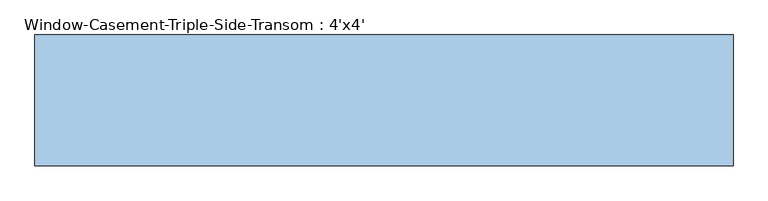
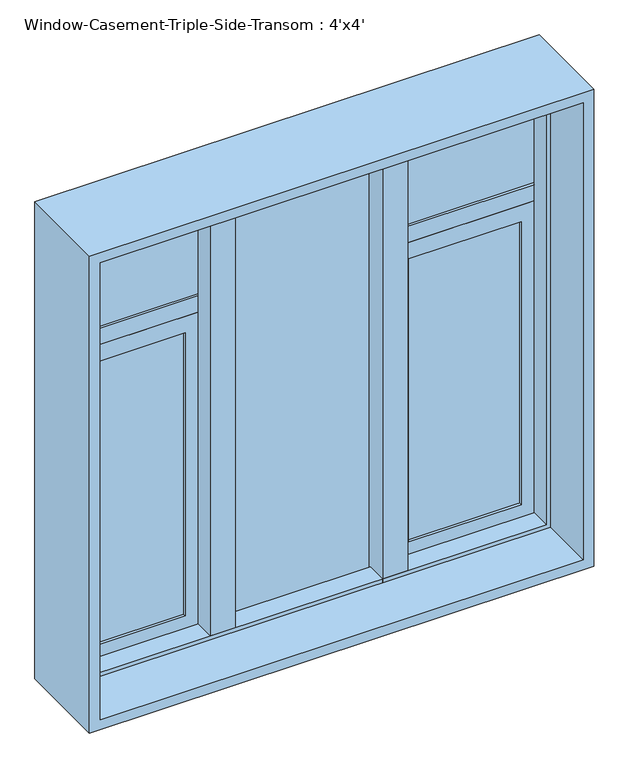
"""IFC4 building model written with IfcOpenShell, lengths in millimetres: window geometry, Window-Casement-Triple-Side-Transom : 4'x4'."""

from ifc_helpers import new_model, si_unit, frame, origin, place, context, project, spatial, polyline, outline, extrude, faceted_brep, source, transform, mapped, element, save


def window_casement_triple_side_transom_4_x4_fd24aed3(model_context):
    return source(origin(), model_context, "Body", "SolidModel", [
        faceted_brep([(-584.2, 73.025, 2108.2), (-584.2, 114.3, 2108.2), (584.2, 114.3, 2108.2), (584.2, 73.025, 2108.2), (-574.0796875, 22.225, 2098.0796875), (-574.0796875, 73.025, 2098.0796875), (574.0796875, 73.025, 2098.0796875), (574.0796875, 22.225, 2098.0796875), (-584.2, -114.3, 2108.2), (-584.2, 22.225, 2108.2), (584.2, 22.225, 2108.2), (584.2, -114.3, 2108.2), (-609.6, 114.3, 2133.6), (-609.6, -114.3, 2133.6), (609.6, -114.3, 2133.6), (609.6, 114.3, 2133.6), (584.2, 114.3, 939.8), (584.2, 73.025, 939.8), (574.0796875, 73.025, 949.9203125), (574.0796875, 22.225, 949.9203125), (584.2, 22.225, 939.8), (584.2, -114.3, 939.8), (609.6, -114.3, 914.4), (609.6, 114.3, 914.4), (-584.2, 114.3, 939.8), (-584.2, 73.025, 939.8), (-574.0796875, 73.025, 949.9203125), (-574.0796875, 22.225, 949.9203125), (-584.2, 22.225, 939.8), (-584.2, -114.3, 939.8), (-609.6, -114.3, 914.4), (-609.6, 114.3, 914.4)], [[[0, 1, 2, 3]], [[4, 5, 6, 7]], [[8, 9, 10, 11]], [[12, 13, 14, 15]], [[3, 2, 16, 17]], [[7, 6, 18, 19]], [[11, 10, 20, 21]], [[15, 14, 22, 23]], [[17, 16, 24, 25]], [[19, 18, 26, 27]], [[21, 20, 28, 29]], [[23, 22, 30, 31]], [[25, 24, 1, 0]], [[3, 17, 25, 0], [5, 26, 18, 6]], [[27, 26, 5, 4]], [[9, 28, 20, 10], [7, 19, 27, 4]], [[29, 28, 9, 8]], [[13, 30, 22, 14], [11, 21, 29, 8]], [[31, 30, 13, 12]], [[15, 23, 31, 12], [1, 24, 16, 2]]]),
        extrude(outline(polyline([(-177.8, 111.125), (-177.8, 22.225), (-238.7203125, 22.225), (-238.7203125, 73.025), (-228.6, 73.025), (-228.6, 111.125), (-177.8, 111.125)])), frame((0.0, 0.0, 939.8), z_axis=(0.0, 0.0, 1.0), x_axis=(1.0, 0.0, 0.0)), (0.0, 0.0, 1.0), 1168.4),
        extrude(outline(polyline([(228.6, 111.125), (228.6, 73.025), (238.7203125, 73.025), (238.7203125, 22.225), (177.8, 22.225), (177.8, 111.125), (228.6, 111.125)])), frame((0.0, 0.0, 939.8), z_axis=(0.0, 0.0, 1.0), x_axis=(1.0, 0.0, 0.0)), (0.0, 0.0, 1.0), 1168.4),
        extrude(outline(polyline([(1746.9048438, 228.6), (939.8, 228.6), (939.8, 584.2), (1746.9048438, 584.2), (1746.9048438, 228.6)]), holes=[polyline([(1705.0345313, 542.3296875), (981.6703125, 542.3296875), (981.6703125, 270.4703125), (1705.0345313, 270.4703125), (1705.0345313, 542.3296875)])]), frame((0.0, 73.025, 0.0), z_axis=(0.0, 1.0, 0.0), x_axis=(0.0, 0.0, 1.0)), (0.0, 0.0, 1.0), 31.75),
        extrude(outline(polyline([(1746.9048438, -584.2), (939.8, -584.2), (939.8, -228.6), (1746.9048438, -228.6), (1746.9048438, -584.2)]), holes=[polyline([(1705.0345313, -270.4703125), (981.6703125, -270.4703125), (981.6703125, -542.3296875), (1705.0345313, -542.3296875), (1705.0345313, -270.4703125)])]), frame((0.0, 73.025, 0.0), z_axis=(0.0, 1.0, 0.0), x_axis=(0.0, 0.0, 1.0)), (0.0, 0.0, 1.0), 31.75),
        extrude(outline(polyline([(-270.4703125, 98.425), (-270.4703125, 92.075), (-542.3296875, 92.075), (-542.3296875, 98.425), (-270.4703125, 98.425)])), frame((0.0, 0.0, 981.6703125), z_axis=(0.0, 0.0, 1.0), x_axis=(1.0, 0.0, 0.0)), (0.0, 0.0, 1.0), 723.3642188),
        extrude(outline(polyline([(-270.4703125, 85.725), (-270.4703125, 79.375), (-542.3296875, 79.375), (-542.3296875, 85.725), (-270.4703125, 85.725)])), frame((0.0, 0.0, 981.6703125), z_axis=(0.0, 0.0, 1.0), x_axis=(1.0, 0.0, 0.0)), (0.0, 0.0, 1.0), 723.3642188),
        extrude(outline(polyline([(542.3296875, 98.425), (542.3296875, 92.075), (270.4703125, 92.075), (270.4703125, 98.425), (542.3296875, 98.425)])), frame((0.0, 0.0, 981.6703125), z_axis=(0.0, 0.0, 1.0), x_axis=(1.0, 0.0, 0.0)), (0.0, 0.0, 1.0), 723.3642188),
        extrude(outline(polyline([(542.3296875, 85.725), (542.3296875, 79.375), (270.4703125, 79.375), (270.4703125, 85.725), (542.3296875, 85.725)])), frame((0.0, 0.0, 981.6703125), z_axis=(0.0, 0.0, 1.0), x_axis=(1.0, 0.0, 0.0)), (0.0, 0.0, 1.0), 723.3642188),
        extrude(outline(polyline([(584.2, 104.775), (584.2, 73.025), (228.6, 73.025), (228.6, 104.775), (584.2, 104.775)])), frame((0.0, 0.0, 1746.9048438), z_axis=(0.0, 0.0, 1.0), x_axis=(1.0, 0.0, 0.0)), (0.0, 0.0, 1.0), 41.8703125),
        extrude(outline(polyline([(177.8, 98.425), (177.8, 92.075), (-177.8, 92.075), (-177.8, 98.425), (177.8, 98.425)])), frame((0.0, 0.0, 939.8), z_axis=(0.0, 0.0, 1.0), x_axis=(1.0, 0.0, 0.0)), (0.0, 0.0, 1.0), 1168.4),
        extrude(outline(polyline([(177.8, 85.725), (177.8, 79.375), (-177.8, 79.375), (-177.8, 85.725), (177.8, 85.725)])), frame((0.0, 0.0, 939.8), z_axis=(0.0, 0.0, 1.0), x_axis=(1.0, 0.0, 0.0)), (0.0, 0.0, 1.0), 1168.4),
        extrude(outline(polyline([(-228.6, 104.775), (-228.6, 73.025), (-584.2, 73.025), (-584.2, 104.775), (-228.6, 104.775)])), frame((0.0, 0.0, 1746.9048438), z_axis=(0.0, 0.0, 1.0), x_axis=(1.0, 0.0, 0.0)), (0.0, 0.0, 1.0), 41.8703125),
        extrude(outline(polyline([(-228.6, 98.425), (-228.6, 92.075), (-584.2, 92.075), (-584.2, 98.425), (-228.6, 98.425)])), frame((0.0, 0.0, 1788.7751562), z_axis=(0.0, 0.0, 1.0), x_axis=(1.0, 0.0, 0.0)), (0.0, 0.0, 1.0), 319.4248438),
        extrude(outline(polyline([(-228.6, 85.725), (-228.6, 79.375), (-584.2, 79.375), (-584.2, 85.725), (-228.6, 85.725)])), frame((0.0, 0.0, 1788.7751562), z_axis=(0.0, 0.0, 1.0), x_axis=(1.0, 0.0, 0.0)), (0.0, 0.0, 1.0), 319.4248438),
        extrude(outline(polyline([(584.2, 98.425), (584.2, 92.075), (228.6, 92.075), (228.6, 98.425), (584.2, 98.425)])), frame((0.0, 0.0, 1788.7751562), z_axis=(0.0, 0.0, 1.0), x_axis=(1.0, 0.0, 0.0)), (0.0, 0.0, 1.0), 319.4248438),
        extrude(outline(polyline([(584.2, 85.725), (584.2, 79.375), (228.6, 79.375), (228.6, 85.725), (584.2, 85.725)])), frame((0.0, 0.0, 1788.7751562), z_axis=(0.0, 0.0, 1.0), x_axis=(1.0, 0.0, 0.0)), (0.0, 0.0, 1.0), 319.4248438),
    ])


if __name__ == "__main__":
    model = new_model("IFC4")
    model_context = context("Model", 3, world=origin())
    ifc_project = project(units=[si_unit("LENGTHUNIT", "METRE", prefix="MILLI")], contexts=[model_context])
    site = spatial("IfcSite", under=ifc_project)
    building = spatial("IfcBuilding", under=site)
    placement = place(None, origin())
    window_casement_triple_side_transom_4_x4_shape = window_casement_triple_side_transom_4_x4_fd24aed3(model_context)
    element("IfcWindow", 1, ObjectType="Window-Casement-Triple-Side-Transom : 4'x4'", at=placement, inside=building, context=model_context, shape_type="MappedRepresentation", body=[
        mapped(window_casement_triple_side_transom_4_x4_shape, transform((0.0, 0.0, 0.0), x_axis=(1.0, 0.0, 0.0), y_axis=(0.0, 1.0, 0.0), z_axis=(0.0, 0.0, 1.0))),
    ])
    save(model, "model.ifc")

# Revit data of these elements
# Type "Window-Casement-Triple-Side-Transom : 4'x4'"
#   Type Mark = "27"
#   Fire Rating = "0.5h"
#   Assembly Code = "B2020100"
#   Analytic Construction = "Double glazing - domestic"
#   Window Width = 1' - 4"
#   Window Inset [instance default] = 0' - 0 5/8"
#   Wall Thickness [instance default] = 0' - 6"
#   Visual Light Transmittance = 0.81
#   Transom Height Ratio = 0.3
#   Thermal Resistance (R) = 1.8146 (h·ft²·°F)/BTU
#   Solar Heat Gain Coefficient = 0.76
#   Rough Width = 4' - 0 1/2"
#   Rough Height = 4' - 0 1/2"
#   Open Window Height = 2' - 9.6"
#   Heat Transfer Coefficient (U) = 0.5511 BTU/(h·ft²·°F)
#   Height = 4' - 0"
#   Transom Height = 1' - 2.4"
#   Frame Gap 3 [instance default] = 0' - 1 83/128"
#   Frame Gap 2 [instance default] = 0' - 0 5/8"
#   Frame Gap 1 = 0' - 1 51/128"
#   Default Sill Height = 3' - 0"
#   Width = 4' - 0"
#   Frame Material = Metal - Aluminum
#   Glass Panel Material = Glass
#   Wall Closure = (empty or 0)
# Element 1 (IfcWindow, "Window-Casement-Triple-Side-Transom : 4'x4'")
#   Wall Thickness = 0' - 9"
#   Materials on its faces: "Metal - Aluminum", "Glass"
# Materials
#   "Metal - Aluminum": class "Metal", colour RGB 247 247 247, transparency 0
#   "Glass": class "Glass", colour RGB 0 128 192, transparency 0.75, Description = "Soda Lime Glass", Cost = 0
